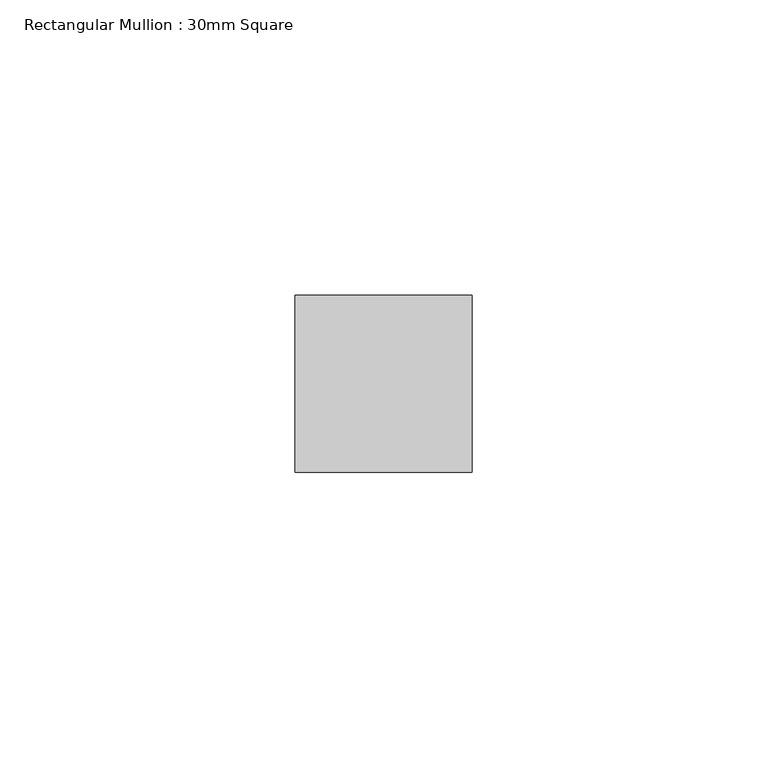
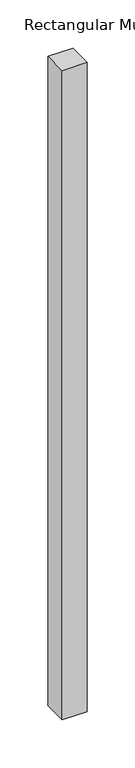
"""IFC4 building model written with IfcOpenShell, lengths in millimetres: member geometry, Rectangular Mullion : 30mm Square."""

from ifc_helpers import new_model, si_unit, frame, origin, place, context, project, spatial, polyline, outline, extrude, source, transform, mapped, element, save


def rectangular_mullion_30mm_square_ca2f0e8b(model_context):
    return source(origin(), model_context, "Body", "SweptSolid", [
        extrude(outline(polyline([(15.0, 15.0), (15.0, -15.0), (-15.0, -15.0), (-15.0, 15.0), (15.0, 15.0)])), frame((0.0, 0.0, -825.0), z_axis=(0.0, 0.0, 1.0), x_axis=(1.0, 0.0, 0.0)), (0.0, 0.0, 1.0), 825.0),
    ])


if __name__ == "__main__":
    model = new_model("IFC4")
    model_context = context("Model", 3, world=origin())
    ifc_project = project(units=[si_unit("LENGTHUNIT", "METRE", prefix="MILLI")], contexts=[model_context])
    site = spatial("IfcSite", under=ifc_project)
    building = spatial("IfcBuilding", under=site)
    placement = place(None, origin())
    rectangular_mullion_30mm_square_shape = rectangular_mullion_30mm_square_ca2f0e8b(model_context)
    element("IfcMember", 1, ObjectType="Rectangular Mullion : 30mm Square", at=placement, inside=building, context=model_context, shape_type="MappedRepresentation", body=[
        mapped(rectangular_mullion_30mm_square_shape, transform((0.0, 0.0, 0.0), x_axis=(1.0, 0.0, 0.0), y_axis=(0.0, 1.0, 0.0), z_axis=(0.0, 0.0, 1.0))),
    ])
    save(model, "model.ifc")

# Revit data of these elements
# Type "Rectangular Mullion : 30mm Square"
#   built-in parameter 1007304 = 0.0984252 (stored number, unit not read)
#   built-in parameter 1007301 = 0.0492126 (stored number, unit not read)
#   built-in parameter 1007300 = 0.0492126 (stored number, unit not read)
# Element 1 (IfcMember, "Rectangular Mullion : 30mm Square")
#   Materials on its faces: "Aluminum"
# Materials
#   "Aluminum": class "Metal", colour RGB 244 244 244, transparency 0, Description = "Aluminum 6061", Cost = 0
